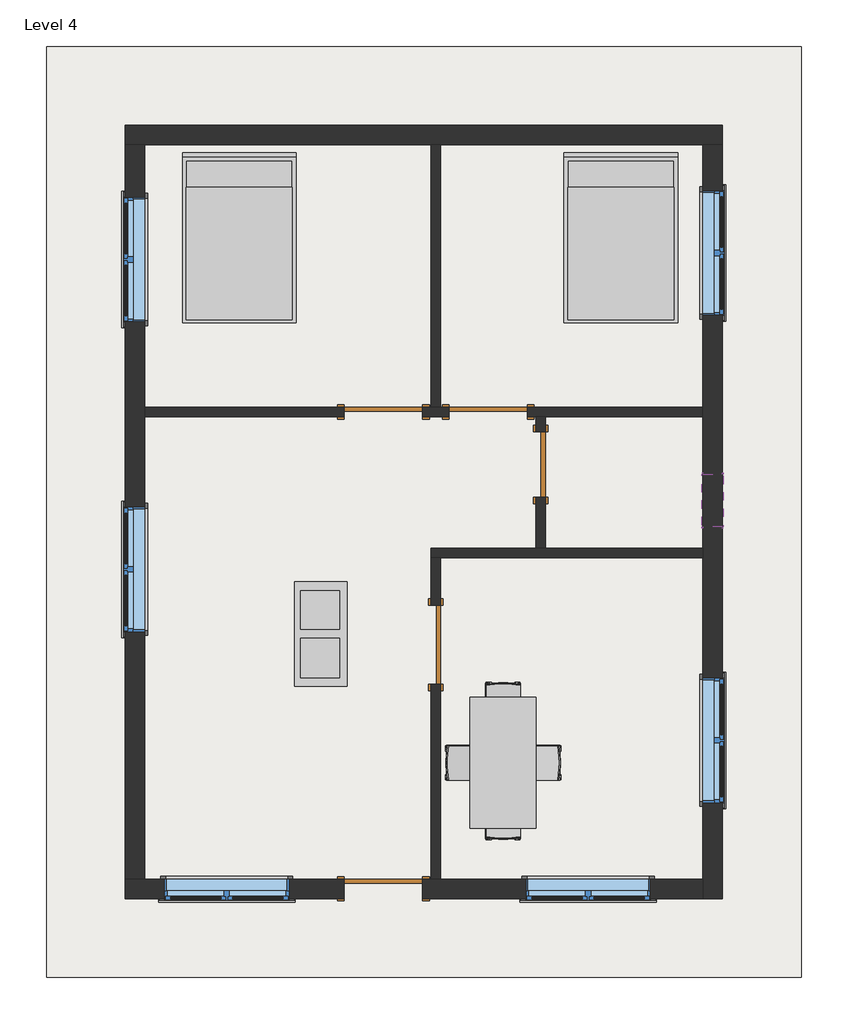
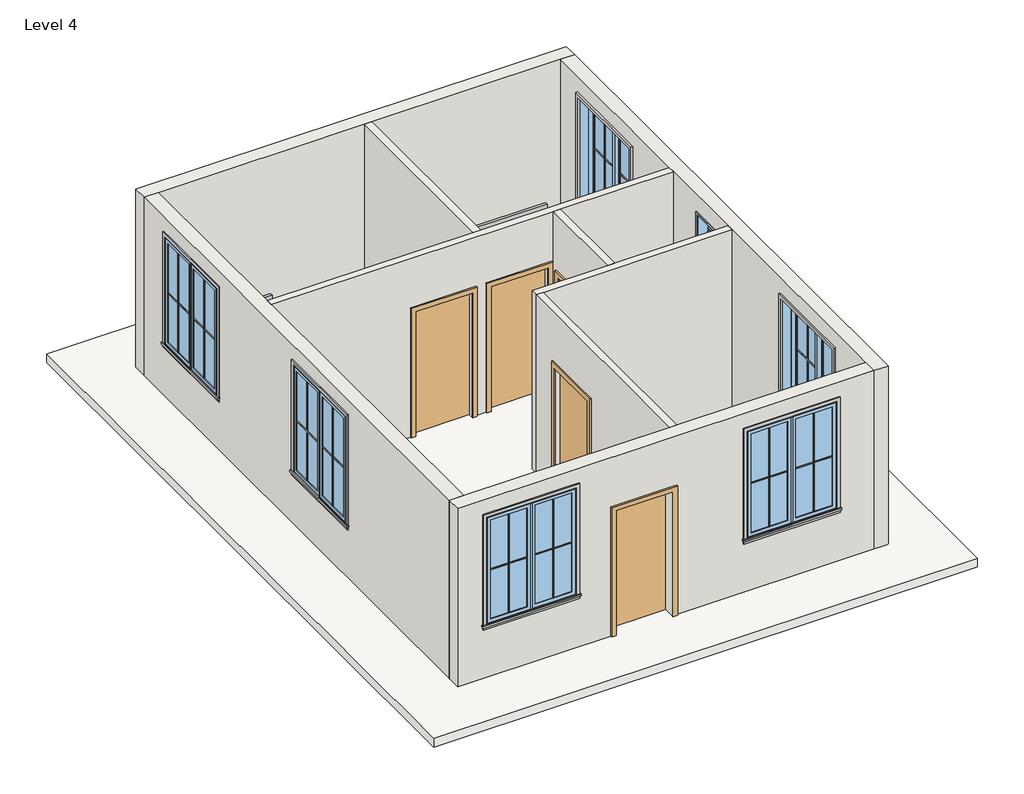
# One storey, incomplete: 25 proxies, 9 walls, 7 windows, 5 doors, 3 furniture elements, 1 roof.
"""IFC4 building model written with IfcOpenShell, lengths in millimetres."""

from ifc_helpers import new_model, si_unit, frame, origin, place, context, project, spatial, polyline, outline, extrude, faceted_brep, transform, mapped, element, save
from components import muntin_pattern_2x2_muntin_pattern_2x2_bff912c5, muntin_pattern_2x2_muntin_pattern_2x2_c2194282, trim_window_exterior_flat_with_sill_e04b3088, trim_window_interior_flat_picture_frame_2a7685fe, coffee_table_with_brass_mullions_11320_coffee_table_with_5962bef7, door_305aa2a5, door_e5f9f3c4, door_0ca8825f, door_f2b275c1, bed_17739_bed_17739_15c61121, dining_table_w_chairs_11374_0cdfc61b, window_9ac97e1a, window_f2d8fef0

model = new_model("IFC4")

# Units and contexts
model_context = context("Model", 3, world=origin())
ifc_project = project(units=[si_unit("LENGTHUNIT", "METRE", prefix="MILLI")], contexts=[model_context])

# Site, building, storey
site = spatial("IfcSite", under=ifc_project)
building = spatial("IfcBuilding", under=site)
storey = spatial("IfcBuildingStorey", under=building, Name="Level 4", Elevation=9448.8)

# Proxies
placement = place(None, origin())
muntin_pattern_2x2_muntin_pattern_2x2_shape = muntin_pattern_2x2_muntin_pattern_2x2_bff912c5(model_context)
element("IfcBuildingElementProxy", 1, Name="Muntin Pattern_2x2 : Muntin Pattern_2x2", ObjectType="Muntin Pattern_2x2 : Muntin Pattern_2x2", at=placement, inside=storey, context=model_context, shape_type="MappedRepresentation", body=[
    mapped(muntin_pattern_2x2_muntin_pattern_2x2_shape, transform((-4718.1437352, -1580.3188735, 10433.05), x_axis=(0.0, 1.0, 0.0), y_axis=(-1.0, 0.0, 0.0), z_axis=(0.0, 0.0, 1.0))),
])
element("IfcBuildingElementProxy", 2, Name="Muntin Pattern_2x2 : Muntin Pattern_2x2", ObjectType="Muntin Pattern_2x2 : Muntin Pattern_2x2", at=placement, inside=storey, context=model_context, shape_type="MappedRepresentation", body=[
    mapped(muntin_pattern_2x2_muntin_pattern_2x2_shape, transform((-3186.2062352, -5039.4813735, 10433.05), x_axis=(-1.0, 0.0, 0.0), y_axis=(0.0, -1.0, 0.0), z_axis=(0.0, 0.0, 1.0))),
])
element("IfcBuildingElementProxy", 3, Name="Muntin Pattern_2x2 : Muntin Pattern_2x2", ObjectType="Muntin Pattern_2x2 : Muntin Pattern_2x2", at=placement, inside=storey, context=model_context, shape_type="MappedRepresentation", body=[
    mapped(muntin_pattern_2x2_muntin_pattern_2x2_shape, transform((1017.4937648, -5039.4813735, 10433.05), x_axis=(-1.0, 0.0, 0.0), y_axis=(0.0, -1.0, 0.0), z_axis=(0.0, 0.0, 1.0))),
])
element("IfcBuildingElementProxy", 4, Name="Muntin Pattern_2x2 : Muntin Pattern_2x2", ObjectType="Muntin Pattern_2x2 : Muntin Pattern_2x2", at=placement, inside=storey, context=model_context, shape_type="MappedRepresentation", body=[
    mapped(muntin_pattern_2x2_muntin_pattern_2x2_shape, transform((2209.7062648, -2847.1438735, 10433.05), x_axis=(0.0, -1.0, 0.0), y_axis=(1.0, 0.0, 0.0), z_axis=(0.0, 0.0, 1.0))),
])
element("IfcBuildingElementProxy", 5, Name="Muntin Pattern_2x2 : Muntin Pattern_2x2", ObjectType="Muntin Pattern_2x2 : Muntin Pattern_2x2", at=placement, inside=storey, context=model_context, shape_type="MappedRepresentation", body=[
    mapped(muntin_pattern_2x2_muntin_pattern_2x2_shape, transform((2209.7062648, 2817.0561265, 10433.05), x_axis=(0.0, -1.0, 0.0), y_axis=(1.0, 0.0, 0.0), z_axis=(0.0, 0.0, 1.0))),
])
element("IfcBuildingElementProxy", 6, Name="Muntin Pattern_2x2 : Muntin Pattern_2x2", ObjectType="Muntin Pattern_2x2 : Muntin Pattern_2x2", at=placement, inside=storey, context=model_context, shape_type="MappedRepresentation", body=[
    mapped(muntin_pattern_2x2_muntin_pattern_2x2_shape, transform((-4718.1437352, 2020.1311265, 10433.05), x_axis=(0.0, 1.0, 0.0), y_axis=(-1.0, 0.0, 0.0), z_axis=(0.0, 0.0, 1.0))),
])
muntin_pattern_2x2_muntin_pattern_2x2_2_shape = muntin_pattern_2x2_muntin_pattern_2x2_c2194282(model_context)
element("IfcBuildingElementProxy", 7, Name="Muntin Pattern_2x2 : Muntin Pattern_2x2", ObjectType="Muntin Pattern_2x2 : Muntin Pattern_2x2", at=placement, inside=storey, context=model_context, shape_type="MappedRepresentation", body=[
    mapped(muntin_pattern_2x2_muntin_pattern_2x2_2_shape, transform((-4718.1437352, -859.5938735, 10433.05), x_axis=(0.0, -1.0, 0.0), y_axis=(1.0, 0.0, 0.0), z_axis=(0.0, 0.0, 1.0))),
])
element("IfcBuildingElementProxy", 8, Name="Muntin Pattern_2x2 : Muntin Pattern_2x2", ObjectType="Muntin Pattern_2x2 : Muntin Pattern_2x2", at=placement, inside=storey, context=model_context, shape_type="MappedRepresentation", body=[
    mapped(muntin_pattern_2x2_muntin_pattern_2x2_2_shape, transform((-3906.9312352, -5039.4813735, 10433.05), x_axis=(1.0, 0.0, 0.0), y_axis=(0.0, 1.0, 0.0), z_axis=(0.0, 0.0, 1.0))),
])
element("IfcBuildingElementProxy", 9, Name="Muntin Pattern_2x2 : Muntin Pattern_2x2", ObjectType="Muntin Pattern_2x2 : Muntin Pattern_2x2", at=placement, inside=storey, context=model_context, shape_type="MappedRepresentation", body=[
    mapped(muntin_pattern_2x2_muntin_pattern_2x2_2_shape, transform((296.7687648, -5039.4813735, 10433.05), x_axis=(1.0, 0.0, 0.0), y_axis=(0.0, 1.0, 0.0), z_axis=(0.0, 0.0, 1.0))),
])
element("IfcBuildingElementProxy", 10, Name="Muntin Pattern_2x2 : Muntin Pattern_2x2", ObjectType="Muntin Pattern_2x2 : Muntin Pattern_2x2", at=placement, inside=storey, context=model_context, shape_type="MappedRepresentation", body=[
    mapped(muntin_pattern_2x2_muntin_pattern_2x2_2_shape, transform((2209.7062648, -3567.8688735, 10433.05), x_axis=(0.0, 1.0, 0.0), y_axis=(-1.0, 0.0, 0.0), z_axis=(0.0, 0.0, 1.0))),
])
element("IfcBuildingElementProxy", 11, Name="Muntin Pattern_2x2 : Muntin Pattern_2x2", ObjectType="Muntin Pattern_2x2 : Muntin Pattern_2x2", at=placement, inside=storey, context=model_context, shape_type="MappedRepresentation", body=[
    mapped(muntin_pattern_2x2_muntin_pattern_2x2_2_shape, transform((2209.7062648, 2096.3311265, 10433.05), x_axis=(0.0, 1.0, 0.0), y_axis=(-1.0, 0.0, 0.0), z_axis=(0.0, 0.0, 1.0))),
])
element("IfcBuildingElementProxy", 12, Name="Muntin Pattern_2x2 : Muntin Pattern_2x2", ObjectType="Muntin Pattern_2x2 : Muntin Pattern_2x2", at=placement, inside=storey, context=model_context, shape_type="MappedRepresentation", body=[
    mapped(muntin_pattern_2x2_muntin_pattern_2x2_2_shape, transform((-4718.1437352, 2740.8561265, 10433.05), x_axis=(0.0, -1.0, 0.0), y_axis=(1.0, 0.0, 0.0), z_axis=(0.0, 0.0, 1.0))),
])
trim_window_exterior_flat_with_sill_shape = trim_window_exterior_flat_with_sill_e04b3088(model_context)
element("IfcBuildingElementProxy", 13, Name="Trim-Window-Exterior-Flat : with Sill", ObjectType="Trim-Window-Exterior-Flat : with Sill", at=placement, inside=storey, context=model_context, shape_type="MappedRepresentation", body=[
    mapped(trim_window_exterior_flat_with_sill_shape, transform((-4727.6687352, -1219.9563735, 12192.0), x_axis=(0.0, -1.0, 0.0), y_axis=(0.0, 0.0, 1.0), z_axis=(-1.0, 0.0, 0.0))),
])
element("IfcBuildingElementProxy", 14, Name="Trim-Window-Exterior-Flat : with Sill", ObjectType="Trim-Window-Exterior-Flat : with Sill", at=placement, inside=storey, context=model_context, shape_type="MappedRepresentation", body=[
    mapped(trim_window_exterior_flat_with_sill_shape, transform((-3546.5687352, -5049.0063735, 12192.0), x_axis=(1.0, 0.0, 0.0), y_axis=(0.0, 0.0, 1.0), z_axis=(0.0, -1.0, 0.0))),
])
element("IfcBuildingElementProxy", 15, Name="Trim-Window-Exterior-Flat : with Sill", ObjectType="Trim-Window-Exterior-Flat : with Sill", at=placement, inside=storey, context=model_context, shape_type="MappedRepresentation", body=[
    mapped(trim_window_exterior_flat_with_sill_shape, transform((657.1312648, -5049.0063735, 12192.0), x_axis=(1.0, 0.0, 0.0), y_axis=(0.0, 0.0, 1.0), z_axis=(0.0, -1.0, 0.0))),
])
element("IfcBuildingElementProxy", 16, Name="Trim-Window-Exterior-Flat : with Sill", ObjectType="Trim-Window-Exterior-Flat : with Sill", at=placement, inside=storey, context=model_context, shape_type="MappedRepresentation", body=[
    mapped(trim_window_exterior_flat_with_sill_shape, transform((2219.2312648, -3207.5063735, 12192.0), x_axis=(0.0, 1.0, 0.0), y_axis=(0.0, 0.0, 1.0), z_axis=(1.0, 0.0, 0.0))),
])
element("IfcBuildingElementProxy", 17, Name="Trim-Window-Exterior-Flat : with Sill", ObjectType="Trim-Window-Exterior-Flat : with Sill", at=placement, inside=storey, context=model_context, shape_type="MappedRepresentation", body=[
    mapped(trim_window_exterior_flat_with_sill_shape, transform((2219.2312648, 2456.6936265, 12192.0), x_axis=(0.0, 1.0, 0.0), y_axis=(0.0, 0.0, 1.0), z_axis=(1.0, 0.0, 0.0))),
])
element("IfcBuildingElementProxy", 18, Name="Trim-Window-Exterior-Flat : with Sill", ObjectType="Trim-Window-Exterior-Flat : with Sill", at=placement, inside=storey, context=model_context, shape_type="MappedRepresentation", body=[
    mapped(trim_window_exterior_flat_with_sill_shape, transform((-4727.6687352, 2380.4936265, 12192.0), x_axis=(0.0, -1.0, 0.0), y_axis=(0.0, 0.0, 1.0), z_axis=(-1.0, 0.0, 0.0))),
])
trim_window_interior_flat_picture_frame_shape = trim_window_interior_flat_picture_frame_2a7685fe(model_context)
element("IfcBuildingElementProxy", 19, Name="Trim-Window-Interior-Flat : Picture Frame", ObjectType="Trim-Window-Interior-Flat : Picture Frame", at=placement, inside=storey, context=model_context, shape_type="MappedRepresentation", body=[
    mapped(trim_window_interior_flat_picture_frame_shape, transform((-4499.0687352, -1219.9563735, 12192.0), x_axis=(0.0, 1.0, 0.0), y_axis=(0.0, 0.0, 1.0), z_axis=(1.0, 0.0, 0.0))),
])
element("IfcBuildingElementProxy", 20, Name="Trim-Window-Interior-Flat : Picture Frame", ObjectType="Trim-Window-Interior-Flat : Picture Frame", at=placement, inside=storey, context=model_context, shape_type="MappedRepresentation", body=[
    mapped(trim_window_interior_flat_picture_frame_shape, transform((-3546.5687352, -4820.4063735, 12192.0), x_axis=(-1.0, 0.0, 0.0), y_axis=(0.0, 0.0, 1.0), z_axis=(0.0, 1.0, 0.0))),
])
element("IfcBuildingElementProxy", 21, Name="Trim-Window-Interior-Flat : Picture Frame", ObjectType="Trim-Window-Interior-Flat : Picture Frame", at=placement, inside=storey, context=model_context, shape_type="MappedRepresentation", body=[
    mapped(trim_window_interior_flat_picture_frame_shape, transform((657.1312648, -4820.4063735, 12192.0), x_axis=(-1.0, 0.0, 0.0), y_axis=(0.0, 0.0, 1.0), z_axis=(0.0, 1.0, 0.0))),
])
element("IfcBuildingElementProxy", 22, Name="Trim-Window-Interior-Flat : Picture Frame", ObjectType="Trim-Window-Interior-Flat : Picture Frame", at=placement, inside=storey, context=model_context, shape_type="MappedRepresentation", body=[
    mapped(trim_window_interior_flat_picture_frame_shape, transform((1990.6312648, -3207.5063735, 12192.0), x_axis=(0.0, -1.0, 0.0), y_axis=(0.0, 0.0, 1.0), z_axis=(-1.0, 0.0, 0.0))),
])
element("IfcBuildingElementProxy", 23, Name="Trim-Window-Interior-Flat : Picture Frame", ObjectType="Trim-Window-Interior-Flat : Picture Frame", at=placement, inside=storey, context=model_context, shape_type="MappedRepresentation", body=[
    mapped(trim_window_interior_flat_picture_frame_shape, transform((1990.6312648, 2456.6936265, 12192.0), x_axis=(0.0, -1.0, 0.0), y_axis=(0.0, 0.0, 1.0), z_axis=(-1.0, 0.0, 0.0))),
])
element("IfcBuildingElementProxy", 24, Name="Trim-Window-Interior-Flat : Picture Frame", ObjectType="Trim-Window-Interior-Flat : Picture Frame", at=placement, inside=storey, context=model_context, shape_type="MappedRepresentation", body=[
    mapped(trim_window_interior_flat_picture_frame_shape, transform((-4499.0687352, 2380.4936265, 12192.0), x_axis=(0.0, 1.0, 0.0), y_axis=(0.0, 0.0, 1.0), z_axis=(1.0, 0.0, 0.0))),
])
coffee_table_with_brass_mullions_11320_coffee_table_with_shape = coffee_table_with_brass_mullions_11320_coffee_table_with_5962bef7(model_context)
element("IfcBuildingElementProxy", 25, Name="coffee_table_with_brass_mullions_11320 : coffee_table_with_brass_mullions_11320", ObjectType="coffee_table_with_brass_mullions_11320 : coffee_table_with_brass_mullions_11320", at=placement, inside=storey, context=model_context, shape_type="MappedRepresentation", body=[
    mapped(coffee_table_with_brass_mullions_11320_coffee_table_with_shape, transform((-2022.5687352, -1334.2563735, 9448.8), x_axis=(0.0, 1.0, 0.0), y_axis=(-1.0, 0.0, 0.0), z_axis=(0.0, 0.0, 1.0))),
])

# Doors
door_shape = door_305aa2a5(model_context)
element("IfcDoor", 26, ObjectType="Single-Flush : 36\" x 84\"", at=placement, inside=storey, context=model_context, shape_type="MappedRepresentation", body=[
    mapped(door_shape, transform((-1114.5187352, -2096.2563735, 9448.8), x_axis=(0.0, 1.0, 0.0), y_axis=(-1.0, 0.0, 0.0), z_axis=(0.0, 0.0, 1.0))),
])
element("IfcDoor", 27, ObjectType="Single-Flush : 36\" x 84\"", at=placement, inside=storey, context=model_context, shape_type="MappedRepresentation", body=[
    mapped(door_shape, transform((-1724.1187352, 608.8436265, 9448.8), x_axis=(-1.0, 0.0, 0.0), y_axis=(0.0, -1.0, 0.0), z_axis=(0.0, 0.0, 1.0))),
])
door_2_shape = door_e5f9f3c4(model_context)
element("IfcDoor", 28, ObjectType="Single-Flush : 36\" x 84\"", at=placement, inside=storey, context=model_context, shape_type="MappedRepresentation", body=[
    mapped(door_2_shape, transform((-504.9187352, 608.8436265, 9448.8), x_axis=(1.0, 0.0, 0.0), y_axis=(0.0, 1.0, 0.0), z_axis=(0.0, 0.0, 1.0))),
])
door_3_shape = door_0ca8825f(model_context)
element("IfcDoor", 29, ObjectType="Single-Flush : 36\" x 84\"", at=placement, inside=storey, context=model_context, shape_type="MappedRepresentation", body=[
    mapped(door_3_shape, transform((-1724.1187352, -4934.7063735, 9448.8), x_axis=(1.0, 0.0, 0.0), y_axis=(0.0, 1.0, 0.0), z_axis=(0.0, 0.0, 1.0))),
])
door_4_shape = door_f2b275c1(model_context)
element("IfcDoor", 30, ObjectType="Single-Flush : DOOR 2'6\"", at=placement, inside=storey, context=model_context, shape_type="MappedRepresentation", body=[
    mapped(door_4_shape, transform((104.6812648, -0.7563735, 9448.8), x_axis=(0.0, 1.0, 0.0), y_axis=(-1.0, 0.0, 0.0), z_axis=(0.0, 0.0, 1.0))),
])

# Furniture
bed_17739_bed_17739_shape = bed_17739_bed_17739_15c61121(model_context)
element("IfcFurniture", 31, ObjectType="Bed_17739 : Bed_17739", at=placement, inside=storey, context=model_context, shape_type="MappedRepresentation", body=[
    mapped(bed_17739_bed_17739_shape, transform((-3400.5187352, 2609.0936265, 9448.8), x_axis=(1.0, 0.0, 0.0), y_axis=(0.0, 1.0, 0.0), z_axis=(0.0, 0.0, 1.0))),
])
element("IfcFurniture", 32, ObjectType="Bed_17739 : Bed_17739", at=placement, inside=storey, context=model_context, shape_type="MappedRepresentation", body=[
    mapped(bed_17739_bed_17739_shape, transform((1038.1312648, 2609.0936265, 9448.8), x_axis=(1.0, 0.0, 0.0), y_axis=(0.0, 1.0, 0.0), z_axis=(0.0, 0.0, 1.0))),
])
dining_table_w_chairs_11374_shape = dining_table_w_chairs_11374_0cdfc61b(model_context)
element("IfcFurniture", 33, ObjectType="Dining_Table_w_Chairs_11374", at=placement, inside=storey, context=model_context, shape_type="MappedRepresentation", body=[
    mapped(dining_table_w_chairs_11374_shape, transform((-238.2576574, -3486.1221401, 9448.8), x_axis=(0.0, 1.0, 0.0), y_axis=(-1.0, 0.0, 0.0), z_axis=(0.0, 0.0, 1.0))),
])

# Roof
element("IfcRoof", 34, ObjectType="ROOF 6\"", at=placement, inside=storey, context=model_context, shape_type="SweptSolid", body=[
    extrude(outline(polyline([(-5642.0687352, 4856.9936265), (3133.6312648, 4856.9936265), (3133.6312648, -5963.4063735), (-5642.0687352, -5963.4063735), (-5642.0687352, 4856.9936265)])), frame((0.0, 0.0, 9296.4), z_axis=(0.0, 0.0, 1.0), x_axis=(1.0, 0.0, 0.0)), (0.0, 0.0, 1.0), 152.4),
])

# Walls
element("IfcWall", 35, ObjectType="WALL 4.5\"", at=placement, inside=storey, context=model_context, shape_type="Brep", body=[
    faceted_brep([(-4499.0687352, 551.6936265, 9448.8), (-2181.3187352, 551.6936265, 9448.8), (-2181.3187352, 551.6936265, 11582.4), (-1266.9187352, 551.6936265, 11582.4), (-1266.9187352, 551.6936265, 9448.8), (-962.1187352, 551.6936265, 9448.8), (-962.1187352, 551.6936265, 11582.4), (-47.7187352, 551.6936265, 11582.4), (-47.7187352, 551.6936265, 9448.8), (47.5312648, 551.6936265, 9448.8), (161.8312648, 551.6936265, 9448.8), (1990.6312648, 551.6936265, 9448.8), (1990.6312648, 551.6936265, 12496.8), (161.8312648, 551.6936265, 12496.8), (47.5312648, 551.6936265, 12496.8), (-4499.0687352, 551.6936265, 12496.8), (-2181.3187352, 665.9936265, 11582.4), (-2181.3187352, 665.9936265, 9448.8), (-4499.0687352, 665.9936265, 9448.8), (-4499.0687352, 665.9936265, 12496.8), (-1171.6687352, 665.9936265, 12496.8), (-1057.3687352, 665.9936265, 12496.8), (1990.6312648, 665.9936265, 12496.8), (1990.6312648, 665.9936265, 9448.8), (-47.7187352, 665.9936265, 9448.8), (-47.7187352, 665.9936265, 11582.4), (-962.1187352, 665.9936265, 11582.4), (-962.1187352, 665.9936265, 9448.8), (-1057.3687352, 665.9936265, 9448.8), (-1171.6687352, 665.9936265, 9448.8), (-1266.9187352, 665.9936265, 9448.8), (-1266.9187352, 665.9936265, 11582.4)], [[[0, 1, 2, 3, 4, 5, 6, 7, 8, 9, 10, 11, 12, 13, 14, 15]], [[16, 17, 18, 19, 20, 21, 22, 23, 24, 25, 26, 27, 28, 29, 30, 31]], [[11, 10, 9, 8, 24, 23]], [[18, 17, 1, 0]], [[30, 29, 28, 27, 5, 4]], [[12, 11, 23, 22]], [[0, 15, 19, 18]], [[25, 24, 8, 7]], [[26, 25, 7, 6]], [[27, 26, 6, 5]], [[2, 1, 17, 16]], [[3, 2, 16, 31]], [[4, 3, 31, 30]], [[15, 14, 13, 12, 22, 21, 20, 19]]]),
])
element("IfcWall", 36, ObjectType="WALL 4.5\"", at=placement, inside=storey, context=model_context, shape_type="SweptSolid", body=[
    extrude(outline(polyline([(-1057.3687352, 3713.9936265), (-1057.3687352, 665.9936265), (-1171.6687352, 665.9936265), (-1171.6687352, 3713.9936265), (-1057.3687352, 3713.9936265)])), frame((0.0, 0.0, 9448.8), z_axis=(0.0, 0.0, 1.0), x_axis=(1.0, 0.0, 0.0)), (0.0, 0.0, 1.0), 3048.0),
])
element("IfcWall", 37, ObjectType="WALL 4.5\"", at=placement, inside=storey, context=model_context, shape_type="Brep", body=[
    faceted_brep([(1990.6312648, -972.3063735, 9448.8), (161.8312648, -972.3063735, 9448.8), (47.5312648, -972.3063735, 9448.8), (-1171.6687352, -972.3063735, 9448.8), (-1171.6687352, -972.3063735, 12496.8), (47.5312648, -972.3063735, 12496.8), (161.8312648, -972.3063735, 12496.8), (1990.6312648, -972.3063735, 12496.8), (1990.6312648, -1086.6063735, 9448.8), (1990.6312648, -1086.6063735, 12496.8), (-1057.3687352, -1086.6063735, 12496.8), (-1171.6687352, -1086.6063735, 12496.8), (-1171.6687352, -1086.6063735, 9448.8), (-1057.3687352, -1086.6063735, 9448.8)], [[[0, 1, 2, 3, 4, 5, 6, 7]], [[8, 9, 10, 11, 12, 13]], [[3, 2, 1, 0, 8, 13, 12]], [[0, 7, 9, 8]], [[4, 3, 12, 11]], [[7, 6, 5, 4, 11, 10, 9]]]),
])
element("IfcWall", 38, ObjectType="WALL 4.5\"", at=placement, inside=storey, context=model_context, shape_type="SweptSolid", body=[
    extrude(outline(polyline([(-1086.6063735, 9448.8), (-1639.0563735, 9448.8), (-1639.0563735, 11582.4), (-2553.4563735, 11582.4), (-2553.4563735, 9448.8), (-4820.4063735, 9448.8), (-4820.4063735, 12496.8), (-1086.6063735, 12496.8), (-1086.6063735, 9448.8)])), frame((-1171.6687352, 0.0, 0.0), z_axis=(1.0, 0.0, 0.0), x_axis=(0.0, 1.0, 0.0)), (0.0, 0.0, 1.0), 114.3),
])
element("IfcWall", 39, ObjectType="WALL 4.5\"", at=placement, inside=storey, context=model_context, shape_type="SweptSolid", body=[
    extrude(outline(polyline([(551.6936265, 9448.8), (380.2436265, 9448.8), (380.2436265, 11480.8), (-381.7563735, 11480.8), (-381.7563735, 9448.8), (-972.3063735, 9448.8), (-972.3063735, 12496.8), (551.6936265, 12496.8), (551.6936265, 9448.8)])), frame((47.5312648, 0.0, 0.0), z_axis=(1.0, 0.0, 0.0), x_axis=(0.0, 1.0, 0.0)), (0.0, 0.0, 1.0), 114.3),
])
element("IfcWall", 40, ObjectType="WALL 9\"", at=placement, inside=storey, context=model_context, shape_type="Brep", body=[
    faceted_brep([(-4727.6687352, 3713.9936265, 9448.8), (-4499.0687352, 3713.9936265, 9448.8), (-1171.6687352, 3713.9936265, 9448.8), (-1057.3687352, 3713.9936265, 9448.8), (1990.6312648, 3713.9936265, 9448.8), (2219.2312648, 3713.9936265, 9448.8), (2219.2312648, 3713.9936265, 12496.8), (1990.6312648, 3713.9936265, 12496.8), (-1057.3687352, 3713.9936265, 12496.8), (-1171.6687352, 3713.9936265, 12496.8), (-4499.0687352, 3713.9936265, 12496.8), (-4727.6687352, 3713.9936265, 12496.8), (-4727.6687352, 3942.5936265, 9448.8), (-4727.6687352, 3942.5936265, 12496.8), (2219.2312648, 3942.5936265, 12496.8), (2219.2312648, 3942.5936265, 9448.8)], [[[0, 1, 2, 3, 4, 5, 6, 7, 8, 9, 10, 11]], [[12, 13, 14, 15]], [[5, 4, 3, 2, 1, 0, 12, 15]], [[6, 5, 15, 14]], [[0, 11, 13, 12]], [[11, 10, 9, 8, 7, 6, 14, 13]]]),
])
element("IfcWall", 41, ObjectType="WALL 9\"", at=placement, inside=storey, context=model_context, shape_type="Brep", body=[
    faceted_brep([(1990.6312648, 3713.9936265, 9448.8), (1990.6312648, 665.9936265, 9448.8), (1990.6312648, 551.6936265, 9448.8), (1990.6312648, -972.3063735, 9448.8), (1990.6312648, -1086.6063735, 9448.8), (1990.6312648, -4820.4063735, 9448.8), (1990.6312648, -5049.0063735, 9448.8), (1990.6312648, -5049.0063735, 12496.8), (1990.6312648, -4820.4063735, 12496.8), (1990.6312648, -1086.6063735, 12496.8), (1990.6312648, -972.3063735, 12496.8), (1990.6312648, 551.6936265, 12496.8), (1990.6312648, 665.9936265, 12496.8), (1990.6312648, 3713.9936265, 12496.8), (1990.6312648, -3931.4063735, 12192.0), (1990.6312648, -3931.4063735, 10363.2), (1990.6312648, -2483.6063735, 10363.2), (1990.6312648, -2483.6063735, 12192.0), (1990.6312648, 1732.7936265, 12192.0), (1990.6312648, 1732.7936265, 10363.2), (1990.6312648, 3180.5936265, 10363.2), (1990.6312648, 3180.5936265, 12192.0), (1990.6312648, -115.0563735, 12192.0), (1990.6312648, -724.6563735, 12192.0), (1990.6312648, -724.6563735, 11582.4), (1990.6312648, -115.0563735, 11582.4), (2219.2312648, 3713.9936265, 9448.8), (2219.2312648, 3713.9936265, 12496.8), (2219.2312648, -5049.0063735, 12496.8), (2219.2312648, -5049.0063735, 9448.8), (2219.2312648, -3931.4063735, 12192.0), (2219.2312648, -2483.6063735, 12192.0), (2219.2312648, -2483.6063735, 10363.2), (2219.2312648, -3931.4063735, 10363.2), (2219.2312648, 1732.7936265, 12192.0), (2219.2312648, 3180.5936265, 12192.0), (2219.2312648, 3180.5936265, 10363.2), (2219.2312648, 1732.7936265, 10363.2), (2219.2312648, -115.0563735, 12192.0), (2219.2312648, -115.0563735, 11582.4), (2219.2312648, -724.6563735, 11582.4), (2219.2312648, -724.6563735, 12192.0)], [[[0, 1, 2, 3, 4, 5, 6, 7, 8, 9, 10, 11, 12, 13], [14, 15, 16, 17], [18, 19, 20, 21], [22, 23, 24, 25]], [[26, 27, 28, 29], [30, 31, 32, 33], [34, 35, 36, 37], [38, 39, 40, 41]], [[6, 5, 4, 3, 2, 1, 0, 26, 29]], [[0, 13, 27, 26]], [[7, 6, 29, 28]], [[15, 14, 30, 33]], [[16, 15, 33, 32]], [[17, 16, 32, 31]], [[14, 17, 31, 30]], [[19, 18, 34, 37]], [[20, 19, 37, 36]], [[21, 20, 36, 35]], [[18, 21, 35, 34]], [[39, 38, 22, 25]], [[40, 39, 25, 24]], [[41, 40, 24, 23]], [[38, 41, 23, 22]], [[13, 12, 11, 10, 9, 8, 7, 28, 27]]]),
])
element("IfcWall", 42, ObjectType="WALL 9\"", at=placement, inside=storey, context=model_context, shape_type="Brep", body=[
    faceted_brep([(1990.6312648, -4820.4063735, 9448.8), (-1057.3687352, -4820.4063735, 9448.8), (-1171.6687352, -4820.4063735, 9448.8), (-1266.9187352, -4820.4063735, 9448.8), (-1266.9187352, -4820.4063735, 11582.4), (-2181.3187352, -4820.4063735, 11582.4), (-2181.3187352, -4820.4063735, 9448.8), (-4499.0687352, -4820.4063735, 9448.8), (-4727.6687352, -4820.4063735, 9448.8), (-4727.6687352, -4820.4063735, 12496.8), (-4499.0687352, -4820.4063735, 12496.8), (-1171.6687352, -4820.4063735, 12496.8), (-1057.3687352, -4820.4063735, 12496.8), (1990.6312648, -4820.4063735, 12496.8), (-4270.4687352, -4820.4063735, 12192.0), (-4270.4687352, -4820.4063735, 10363.2), (-2822.6687352, -4820.4063735, 10363.2), (-2822.6687352, -4820.4063735, 12192.0), (-66.7687352, -4820.4063735, 12192.0), (-66.7687352, -4820.4063735, 10363.2), (1381.0312648, -4820.4063735, 10363.2), (1381.0312648, -4820.4063735, 12192.0), (-1266.9187352, -5049.0063735, 11582.4), (-1266.9187352, -5049.0063735, 9448.8), (1990.6312648, -5049.0063735, 9448.8), (1990.6312648, -5049.0063735, 12496.8), (-4727.6687352, -5049.0063735, 12496.8), (-4727.6687352, -5049.0063735, 9448.8), (-2181.3187352, -5049.0063735, 9448.8), (-2181.3187352, -5049.0063735, 11582.4), (-4270.4687352, -5049.0063735, 12192.0), (-2822.6687352, -5049.0063735, 12192.0), (-2822.6687352, -5049.0063735, 10363.2), (-4270.4687352, -5049.0063735, 10363.2), (-66.7687352, -5049.0063735, 12192.0), (1381.0312648, -5049.0063735, 12192.0), (1381.0312648, -5049.0063735, 10363.2), (-66.7687352, -5049.0063735, 10363.2)], [[[0, 1, 2, 3, 4, 5, 6, 7, 8, 9, 10, 11, 12, 13], [14, 15, 16, 17], [18, 19, 20, 21]], [[22, 23, 24, 25, 26, 27, 28, 29], [30, 31, 32, 33], [34, 35, 36, 37]], [[28, 27, 8, 7, 6]], [[24, 23, 3, 2, 1, 0]], [[0, 13, 25, 24]], [[9, 8, 27, 26]], [[15, 14, 30, 33]], [[16, 15, 33, 32]], [[17, 16, 32, 31]], [[14, 17, 31, 30]], [[19, 18, 34, 37]], [[20, 19, 37, 36]], [[21, 20, 36, 35]], [[18, 21, 35, 34]], [[4, 3, 23, 22]], [[5, 4, 22, 29]], [[6, 5, 29, 28]], [[13, 12, 11, 10, 9, 26, 25]]]),
])
element("IfcWall", 43, ObjectType="WALL 9\"", at=placement, inside=storey, context=model_context, shape_type="Brep", body=[
    faceted_brep([(-4499.0687352, -4820.4063735, 9448.8), (-4499.0687352, 551.6936265, 9448.8), (-4499.0687352, 665.9936265, 9448.8), (-4499.0687352, 3713.9936265, 9448.8), (-4499.0687352, 3713.9936265, 12496.8), (-4499.0687352, 665.9936265, 12496.8), (-4499.0687352, 551.6936265, 12496.8), (-4499.0687352, -4820.4063735, 12496.8), (-4499.0687352, -496.0563735, 12192.0), (-4499.0687352, -496.0563735, 10363.2), (-4499.0687352, -1943.8563735, 10363.2), (-4499.0687352, -1943.8563735, 12192.0), (-4499.0687352, 3104.3936265, 12192.0), (-4499.0687352, 3104.3936265, 10363.2), (-4499.0687352, 1656.5936265, 10363.2), (-4499.0687352, 1656.5936265, 12192.0), (-4727.6687352, -4820.4063735, 9448.8), (-4727.6687352, -4820.4063735, 12496.8), (-4727.6687352, 3713.9936265, 12496.8), (-4727.6687352, 3713.9936265, 9448.8), (-4727.6687352, -496.0563735, 12192.0), (-4727.6687352, -1943.8563735, 12192.0), (-4727.6687352, -1943.8563735, 10363.2), (-4727.6687352, -496.0563735, 10363.2), (-4727.6687352, 3104.3936265, 12192.0), (-4727.6687352, 1656.5936265, 12192.0), (-4727.6687352, 1656.5936265, 10363.2), (-4727.6687352, 3104.3936265, 10363.2)], [[[0, 1, 2, 3, 4, 5, 6, 7], [8, 9, 10, 11], [12, 13, 14, 15]], [[16, 17, 18, 19], [20, 21, 22, 23], [24, 25, 26, 27]], [[3, 2, 1, 0, 16, 19]], [[4, 3, 19, 18]], [[0, 7, 17, 16]], [[9, 8, 20, 23]], [[10, 9, 23, 22]], [[11, 10, 22, 21]], [[8, 11, 21, 20]], [[13, 12, 24, 27]], [[14, 13, 27, 26]], [[15, 14, 26, 25]], [[12, 15, 25, 24]], [[7, 6, 5, 4, 18, 17]]]),
])

# Windows
window_shape = window_9ac97e1a(model_context)
element("IfcWindow", 44, ObjectType="Window-Casement-Double : 57\" x 72\"", at=placement, inside=storey, context=model_context, shape_type="MappedRepresentation", body=[
    mapped(window_shape, transform((-4613.3687352, -1219.9563735, 9448.8), x_axis=(0.0, 1.0, 0.0), y_axis=(-1.0, 0.0, 0.0), z_axis=(0.0, 0.0, 1.0))),
])
element("IfcWindow", 45, ObjectType="Window-Casement-Double : 57\" x 72\"", at=placement, inside=storey, context=model_context, shape_type="MappedRepresentation", body=[
    mapped(window_shape, transform((-3546.5687352, -4934.7063735, 9448.8), x_axis=(-1.0, 0.0, 0.0), y_axis=(0.0, -1.0, 0.0), z_axis=(0.0, 0.0, 1.0))),
])
element("IfcWindow", 46, ObjectType="Window-Casement-Double : 57\" x 72\"", at=placement, inside=storey, context=model_context, shape_type="MappedRepresentation", body=[
    mapped(window_shape, transform((657.1312648, -4934.7063735, 9448.8), x_axis=(-1.0, 0.0, 0.0), y_axis=(0.0, -1.0, 0.0), z_axis=(0.0, 0.0, 1.0))),
])
element("IfcWindow", 47, ObjectType="Window-Casement-Double : 57\" x 72\"", at=placement, inside=storey, context=model_context, shape_type="MappedRepresentation", body=[
    mapped(window_shape, transform((2104.9312648, -3207.5063735, 9448.8), x_axis=(0.0, -1.0, 0.0), y_axis=(1.0, 0.0, 0.0), z_axis=(0.0, 0.0, 1.0))),
])
element("IfcWindow", 48, ObjectType="Window-Casement-Double : 57\" x 72\"", at=placement, inside=storey, context=model_context, shape_type="MappedRepresentation", body=[
    mapped(window_shape, transform((2104.9312648, 2456.6936265, 9448.8), x_axis=(0.0, -1.0, 0.0), y_axis=(1.0, 0.0, 0.0), z_axis=(0.0, 0.0, 1.0))),
])
element("IfcWindow", 49, ObjectType="Window-Casement-Double : 57\" x 72\"", at=placement, inside=storey, context=model_context, shape_type="MappedRepresentation", body=[
    mapped(window_shape, transform((-4613.3687352, 2380.4936265, 9448.8), x_axis=(0.0, 1.0, 0.0), y_axis=(-1.0, 0.0, 0.0), z_axis=(0.0, 0.0, 1.0))),
])
window_2_shape = window_f2d8fef0(model_context)
element("IfcWindow", 50, ObjectType="Window-Louvers : 24\" x 24\"", at=placement, inside=storey, context=model_context, shape_type="MappedRepresentation", body=[
    mapped(window_2_shape, transform((2111.2812648, -419.8563735, 10668.0), x_axis=(0.0, -1.0, 0.0), y_axis=(1.0, 0.0, 0.0), z_axis=(0.0, 0.0, 1.0))),
])

save(model, "model.ifc")

# Revit data of these elements
# Type "Muntin Pattern_2x2 : Muntin Pattern_2x2"
#   Width [instance default] = 4' - 0"
#   Thickness = 0' - 0 1/2"
#   Height [instance default] = 4' - 0"
#   Distance = 0' - 0 3/4"
#   Interior Material [instance default] = none
#   Exterior Material [instance default] = none
#   Default Elevation = 0
# Type "Trim-Window-Exterior-Flat : with Sill"
#   Trim Width = 0' - 2 1/4"
#   Trim Thickness_Picture Frame = 0' - 1 1/4"
#   Trim Thickness_with Sill = 0' - 0 3/4"
#   Sill Thickness = 0' - 1 1/4"
#   Opening Width [instance default] = 2' - 0"
#   Opening Height [instance default] = 3' - 0"
#   Default Elevation = 4' - 0"
#   Sill = yes
#   Picture Frame = no
#   Trim Material [instance default] = none
# Type "Trim-Window-Interior-Flat : Picture Frame"
#   Trim Thickness_Picture Frame = 0' - 1 1/4"
#   Trim Width = 0' - 2 1/4"
#   Trim Thickness_with Sill = 0' - 0 3/4"
#   Sill Thickness = 0' - 1 1/4"
#   Opening Width [instance default] = 2' - 0"
#   Opening Height [instance default] = 3' - 0"
#   Default Elevation = 4' - 0"
#   Sill = no
#   Picture Frame = yes
#   Trim Material [instance default] = none
# Type "coffee_table_with_brass_mullions_11320 : coffee_table_with_brass_mullions_11320"
#   Default Elevation = 0
# Type "Single-Flush : 36\" x 84\""
#   Type Mark = "1"
#   Construction Type Id = "MDOOR"
#   Assembly Code = "C1020"
#   Analytic Construction = "Metal"
#   Thickness = 0' - 2"
#   Heat Transfer Coefficient (U) = 0.651978 BTU/(h·ft²·°F)
#   Height = 7' - 0"
#   Trim Projection Ext = 0' - 1"
#   Trim Projection Int = 0' - 1"
#   Trim Width = 0' - 3"
#   Width = 3' - 0"
#   Define Thermal Properties by = 1
#   Define Thermal Properties by = 1
#   Door Material = Door - Panel
#   Frame Material = Door - Frame
#   Visual Light Transmittance = 0
#   Solar Heat Gain Coefficient = 0
#   Function = (empty or 0)
#   Wall Closure = (empty or 0)
# Type "Single-Flush : DOOR 2'6\""
#   Type Mark = "8"
#   Construction Type Id = "MDOOR"
#   Assembly Code = "C1020"
#   Analytic Construction = "Metal"
#   Thickness = 0' - 2"
#   Heat Transfer Coefficient (U) = 0.651978 BTU/(h·ft²·°F)
#   Height = 6' - 8"
#   Trim Projection Ext = 0' - 1"
#   Trim Projection Int = 0' - 1"
#   Trim Width = 0' - 3"
#   Width = 2' - 6"
#   Define Thermal Properties by = 1
#   Door Material = Door - Panel
#   Frame Material = Door - Frame
#   Visual Light Transmittance = 0
#   Solar Heat Gain Coefficient = 0
#   Function = (empty or 0)
#   Wall Closure = (empty or 0)
# Type "Bed_17739 : Bed_17739"
#   Default Elevation = 0
# Type "Dining_Table_w_Chairs_11374"
#   Default Elevation = 0
#   Assembly Code = ""
# Type "ROOF 6\""
#   Assembly Code = "B1020"
#   Layers, outside or top first: 0' - 6" no material (function 1)
# Type "WALL 4.5\""
#   Assembly Code = "B2010"
#   Layers, outside or top first: 0' - 4 1/2" no material (function 1)
# Type "WALL 9\""
#   Assembly Code = "B2010"
#   Layers, outside or top first: 0' - 9" no material (function 1)
# Type "Window-Casement-Double : 57\" x 72\""
#   Type Mark = "17"
#   Fire Rating = "0.5h"
#   Assembly Code = "B2020100"
#   Analytic Construction = "Double glazing - domestic"
#   Frame Extension [instance default] = 0' - 0 1/4"
#   Window Inset [instance default] = 0' - 0"
#   Wall Thickness [instance default] = 0' - 6"
#   Interior Wall Closure [instance default] = 0' - 2 1/4"
#   Half Width = 2' - 4 1/2"
#   Visual Light Transmittance = 0.81
#   Thermal Resistance (R) = 1.8146 (h·ft²·°F)/BTU
#   Solar Heat Gain Coefficient = 0.76
#   Rough Width = 4' - 9 1/2"
#   Rough Height = 6' - 0 1/2"
#   Height = 6' - 0"
#   Heat Transfer Coefficient (U) = 0.5511 BTU/(h·ft²·°F)
#   Exterior Wall Closure [instance default] = 0' - 1 1/4"
#   Extension Jamb [instance default] = 0' - 2 1/4"
#   Default Sill Height = 3' - 0"
#   Width = 4' - 9"
#   Define Thermal Properties by = 0
#   Muntin Visibility = yes
#   Interior Trim Visibility [instance default] = yes
#   Exterior Trim Visibility [instance default] = yes
#   Extension Jamb Visibility [instance default] = yes
#   Interior Trim Material = Wood - Stained
#   Muntin Pattern = Muntin Pattern_2x2 : Muntin Pattern_2x2
#   Interior Trim = Trim-Window-Interior-Flat : Picture Frame
#   Interior Frame Material = Wood - Stained
#   Glass Panel Material = Glass
#   Exterior Trim Material = Clad - White
#   Exterior Trim = Trim-Window-Exterior-Flat : with Sill
#   Exterior Frame Material = Clad - White
#   Wall Closure = (empty or 0)
# Type "Window-Louvers : 24\" x 24\""
#   Type Mark = "18"
#   Construction Type Id = "GSP4R"
#   Assembly Code = "B20"
#   Analytic Construction = "1/8 in Pilkington single glazing"
#   Visual Light Transmittance = 0.9
#   Thermal Resistance (R) = 1.53941 (h·ft²·°F)/BTU
#   Solar Heat Gain Coefficient = 0.78
#   Max Height = 1' - 11.74264"
#   Height = 2' - 0"
#   Heat Transfer Coefficient (U) = 0.6496 BTU/(h·ft²·°F)
#   Blade Width [instance default] = 1' - 10 1/2"
#   Blade Vertical Thickness = 0' - 0.35355"
#   Blade Thickness = 0' - 0 1/4"
#   Blade Spacing = 0' - 1 1/2"
#   Blade Height = 0' - 1.85355"
#   Blade Depth = 0' - 3"
#   Blade Angle = 45.00°
#   Default Sill Height = 3' - 0"
#   Trim Projection_Exterior = 0' - 0 1/2"
#   Trim Projection_Interior = 0' - 0 1/2"
#   Trim Width_Exterior = 0' - 1 1/2"
#   Trim Width_Interior = 0' - 1 1/2"
#   Width = 2' - 0"
#   Max Blade Count = 12
#   Define Thermal Properties by = 1
#   Blade Count = 12
#   Frame Material = Birch
#   Louver Material = Birch
#   Trim Exterior Material = Birch
#   Trim Interior Material = Birch
#   Wall Closure = (empty or 0)
# Elements 1, 2, 3, 4, 5, 6, 7, 8, 9, 10, 11, 12 (IfcBuildingElementProxy, "Muntin Pattern_2x2 : Muntin Pattern_2x2")
#   Width = 1' - 11 1/8"
#   Height = 5' - 6 1/2"
#   Interior Material = Wood - Stained
#   Exterior Material = Clad - White
#   Phase Created = New Construction
#   Materials on its faces: "Clad - White", "Wood - Stained"
# Elements 13, 14, 15, 16, 17, 18 (IfcBuildingElementProxy, "Trim-Window-Exterior-Flat : with Sill")
#   Opening Width = 4' - 9"
#   Opening Height = 6' - 0"
#   Trim Material = Clad - White
#   Phase Created = New Construction
#   Materials on its faces: "Clad - White"
# Elements 19, 20, 21, 22, 23, 24 (IfcBuildingElementProxy, "Trim-Window-Interior-Flat : Picture Frame")
#   Opening Width = 4' - 9"
#   Opening Height = 6' - 0"
#   Trim Material = Wood - Stained
#   Phase Created = New Construction
#   Materials on its faces: "Wood - Stained"
# Element 25 (IfcBuildingElementProxy, "coffee_table_with_brass_mullions_11320 : coffee_table_with_brass_mullions_11320")
#   Phase Created = New Construction
#   Materials on its faces: "Default Wall", "TABLE", "Glass", "Default"
# Elements 26, 27, 28, 29 (IfcDoor, "Single-Flush : 36\" x 84\"")
#   Phase Created = New Construction
#   Materials on its faces: "Door - Frame", "Door - Panel"
# Element 30 (IfcDoor, "Single-Flush : DOOR 2'6\"")
#   Phase Created = New Construction
#   Materials on its faces: "Door - Frame", "Door - Panel"
# Elements 31, 32 (IfcFurniture, "Bed_17739 : Bed_17739")
#   Phase Created = New Construction
#   Materials on its faces: "legs", "sheets", "bed frame", "Blanket"
# Element 33 (IfcFurniture, "Dining_Table_w_Chairs_11374")
#   Phase Created = New Construction
# Element 34 (IfcRoof, "ROOF 6\"")
#   built-in parameter 1001705 = 31 (stored number, unit not read)
#   built-in parameter 1001701 = -0.5 (stored number, unit not read)
#   built-in parameter 1001710 = 33615
#   Phase Created = New Construction
#   Materials on its faces: "Copper", "Default Roof", "Wood - Stained"
# Elements 35, 36, 37, 38, 39 (IfcWall, "WALL 4.5\"")
#   Top Offset = 0' - 0"
#   Base Offset = 0' - 0"
#   Unconnected Height = 10' - 0"
#   wall height = 10' - 0"
#   Phase Created = New Construction
#   Base Constraint = Level 4
#   Materials on its faces: "Default Wall"
# Elements 40, 41, 42, 43 (IfcWall, "WALL 9\"")
#   Top Offset = 0' - 0"
#   Base Offset = 0' - 0"
#   Unconnected Height = 10' - 0"
#   wall height = 10' - 0"
#   Phase Created = New Construction
#   Base Constraint = Level 4
#   Materials on its faces: "Default Wall", "Parking Stripe"
# Element 44 (IfcWindow, "Window-Casement-Double : 57\" x 72\"")
#   Mark = "22"
#   Window Inset = 0' - 0"
#   Interior Wall Closure = 0' - 2 1/4"
#   Frame Extension = 0' - 0 1/4"
#   Exterior Wall Closure = 0' - 1 1/4"
#   Interior Trim Visibility = yes
#   Exterior Trim Visibility = yes
#   Phase Created = New Construction
#   Materials on its faces: "Wood - Stained", "Glass", "Clad - White"
# Element 45 (IfcWindow, "Window-Casement-Double : 57\" x 72\"")
#   Mark = "23"
#   Window Inset = 0' - 0"
#   Interior Wall Closure = 0' - 2 1/4"
#   Frame Extension = 0' - 0 1/4"
#   Exterior Wall Closure = 0' - 1 1/4"
#   Interior Trim Visibility = yes
#   Exterior Trim Visibility = yes
#   Phase Created = New Construction
#   Materials on its faces: "Wood - Stained", "Glass", "Clad - White"
# Element 46 (IfcWindow, "Window-Casement-Double : 57\" x 72\"")
#   Mark = "24"
#   Window Inset = 0' - 0"
#   Interior Wall Closure = 0' - 2 1/4"
#   Frame Extension = 0' - 0 1/4"
#   Exterior Wall Closure = 0' - 1 1/4"
#   Interior Trim Visibility = yes
#   Exterior Trim Visibility = yes
#   Phase Created = New Construction
#   Materials on its faces: "Wood - Stained", "Glass", "Clad - White"
# Element 47 (IfcWindow, "Window-Casement-Double : 57\" x 72\"")
#   Mark = "25"
#   Window Inset = 0' - 0"
#   Interior Wall Closure = 0' - 2 1/4"
#   Frame Extension = 0' - 0 1/4"
#   Exterior Wall Closure = 0' - 1 1/4"
#   Interior Trim Visibility = yes
#   Exterior Trim Visibility = yes
#   Phase Created = New Construction
#   Materials on its faces: "Wood - Stained", "Glass", "Clad - White"
# Element 48 (IfcWindow, "Window-Casement-Double : 57\" x 72\"")
#   Mark = "26"
#   Window Inset = 0' - 0"
#   Interior Wall Closure = 0' - 2 1/4"
#   Frame Extension = 0' - 0 1/4"
#   Exterior Wall Closure = 0' - 1 1/4"
#   Interior Trim Visibility = yes
#   Exterior Trim Visibility = yes
#   Phase Created = New Construction
#   Materials on its faces: "Wood - Stained", "Glass", "Clad - White"
# Element 49 (IfcWindow, "Window-Casement-Double : 57\" x 72\"")
#   Mark = "27"
#   Window Inset = 0' - 0"
#   Interior Wall Closure = 0' - 2 1/4"
#   Frame Extension = 0' - 0 1/4"
#   Exterior Wall Closure = 0' - 1 1/4"
#   Interior Trim Visibility = yes
#   Exterior Trim Visibility = yes
#   Phase Created = New Construction
#   Materials on its faces: "Wood - Stained", "Glass", "Clad - White"
# Element 50 (IfcWindow, "Window-Louvers : 24\" x 24\"")
#   Mark = "28"
#   Blade Width = 1' - 10 1/2"
#   Phase Created = New Construction
#   Materials on its faces: "Birch"
# Materials
#   "Door - Panel": class "Wood", colour RGB 210 159 95, transparency 0, Cost = 0
#   "Door - Frame": colour RGB 118 70 51, transparency 0, Cost = 0
#   "Wood - Stained": class "Wood", colour RGB 224 178 126, transparency 0, Cost = 0
#   "Glass": class "Glass", colour RGB 0 128 192, transparency 0.75, Description = "Soda Lime Glass", Cost = 0
#   "Clad - White": class "Wood", colour RGB 242 242 238, transparency 0, Cost = 0
#   "Birch": class "Wood", colour RGB 224 178 126, transparency 0, Description = "Betula Alleghaniensis", Cost = 0
#   "Default Wall": colour RGB 128 128 128, transparency 0, Cost = 0
#   "TABLE": class "Generic", colour RGB 120 120 120, transparency 0, Cost = 0
#   "Default": colour RGB 127 127 127, transparency 0, Cost = 0
#   "legs": colour RGB 90 73 37, transparency 0, Cost = 0
#   "sheets": colour RGB 200 195 176, transparency 0, Cost = 0
#   "bed frame": colour RGB 90 73 37, transparency 0, Cost = 0
#   "Blanket": class "System", colour RGB 59 0 1, transparency 0, Cost = 0
#   "Copper": class "Metal", colour RGB 0 0 0, transparency 0, Description = "Copper, matte finish", Cost = 0
#   "Default Roof": colour RGB 88 101 114, transparency 0, Cost = 0
#   "Parking Stripe": class "Paint", colour RGB 250 250 91, transparency 0, Cost = 0
